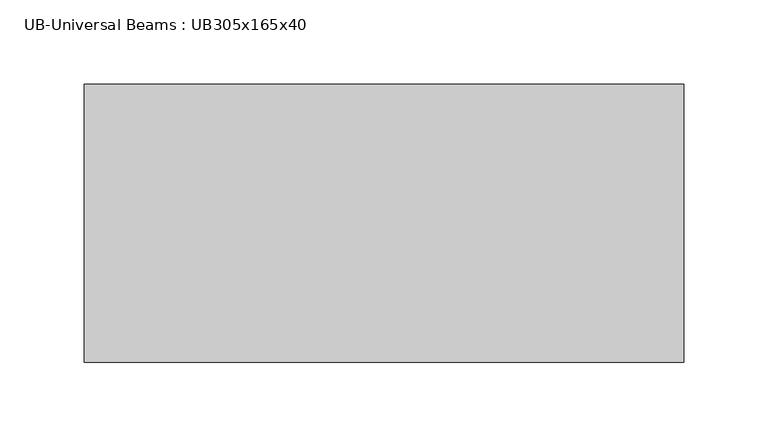
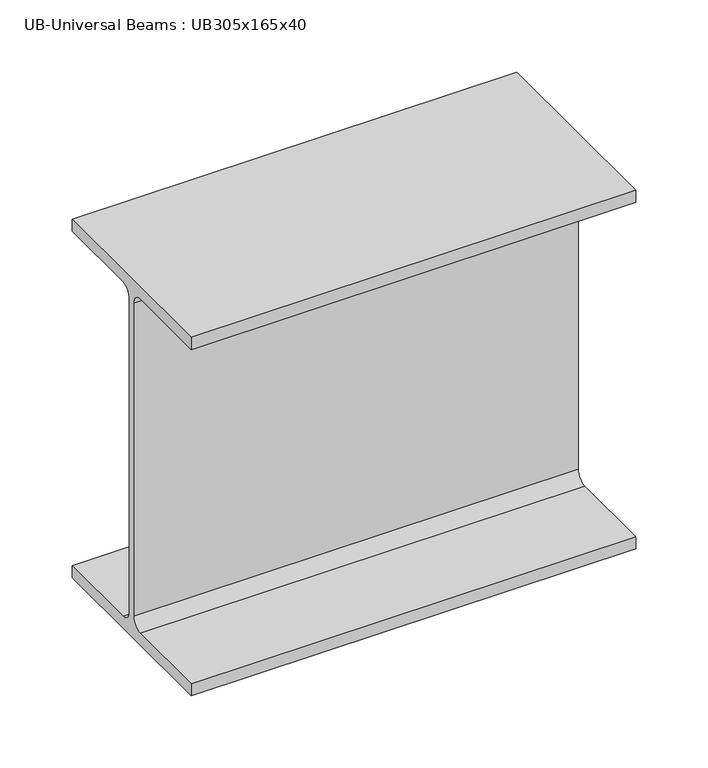
"""IFC4 building model written with IfcOpenShell, lengths in millimetres: beam geometry, UB-Universal Beams : UB305x165x40."""

from ifc_helpers import new_model, si_unit, point, frame, frame_2d, origin, place, context, project, spatial, polyline, circle_curve, trimmed, segment, composite_curve, outline, extrude, source, transform, mapped, element, save


def ub_universal_beams_ub305x165x40_d145b1f7(model_context):
    return source(origin(), model_context, "Body", "SweptSolid", [
        extrude(outline(composite_curve([segment(polyline([(-82.5, -141.5), (-11.9, -141.5)]), True, "CONTINUOUS"), segment(trimmed(circle_curve(frame_2d((-11.9, -132.6)), 8.9), [point((-11.9, -141.5))], [point((-3.0, -132.6))], True, "CARTESIAN"), True, "CONTINUOUS"), segment(polyline([(-3.0, -132.6), (-3.0, 132.6)]), True, "CONTINUOUS"), segment(trimmed(circle_curve(frame_2d((-11.9, 132.6)), 8.9), [point((-3.0, 132.6))], [point((-11.9, 141.5))], True, "CARTESIAN"), True, "CONTINUOUS"), segment(polyline([(-11.9, 141.5), (-82.5, 141.5), (-82.5, 151.7), (82.5, 151.7), (82.5, 141.5), (11.9, 141.5)]), True, "CONTINUOUS"), segment(trimmed(circle_curve(frame_2d((11.9, 132.6)), 8.9), [point((11.9, 141.5))], [point((3.0, 132.6))], True, "CARTESIAN"), True, "CONTINUOUS"), segment(polyline([(3.0, 132.6), (3.0, -132.6)]), True, "CONTINUOUS"), segment(trimmed(circle_curve(frame_2d((11.9, -132.6)), 8.9), [point((3.0, -132.6))], [point((11.9, -141.5))], True, "CARTESIAN"), True, "CONTINUOUS"), segment(polyline([(11.9, -141.5), (82.5, -141.5), (82.5, -151.7), (-82.5, -151.7), (-82.5, -141.5)]), True, "CONTINUOUS")], self_intersect=False)), frame((-665.55, 0.0, 0.0), z_axis=(1.0, 0.0, 0.0), x_axis=(0.0, 1.0, 0.0)), (0.0, 0.0, 1.0), 355.9),
    ])


if __name__ == "__main__":
    model = new_model("IFC4")
    model_context = context("Model", 3, world=origin())
    ifc_project = project(units=[si_unit("LENGTHUNIT", "METRE", prefix="MILLI")], contexts=[model_context])
    site = spatial("IfcSite", under=ifc_project)
    building = spatial("IfcBuilding", under=site)
    placement = place(None, origin())
    ub_universal_beams_ub305x165x40_shape = ub_universal_beams_ub305x165x40_d145b1f7(model_context)
    element("IfcBeam", 1, ObjectType="UB-Universal Beams : UB305x165x40", at=placement, inside=building, context=model_context, shape_type="MappedRepresentation", body=[
        mapped(ub_universal_beams_ub305x165x40_shape, transform((0.0, 0.0, 0.0), x_axis=(1.0, 0.0, 0.0), y_axis=(0.0, 1.0, 0.0), z_axis=(0.0, 0.0, 1.0))),
    ])
    save(model, "model.ifc")

# Revit data of these elements
# Type "UB-Universal Beams : UB305x165x40"
#   Section Name Key = "UB305X165X40"
#   Width = 16.5 cm
#   Web Thickness = 0.6 cm
#   Web Fillet = 0.89 cm
#   Warping Constant = 164000.0 cm⁶
#   Torsional Moment of Inertia = 14.70 cm⁴
#   Section Area = 51.3 cm²
#   Plastic Modulus weak axis = 142.0 cm³
#   Plastic Modulus strong axis = 623.0 cm³
#   Nominal Weight = 40.2999 kgf/m
#   Moment of Inertia weak axis = 764.00 cm⁴
#   Moment of Inertia strong axis = 8503.00 cm⁴
#   Height = 30.34 cm
#   Flange Thickness = 1.02 cm
#   Elastic Modulus weak axis = 92.6 cm³
#   Elastic Modulus strong axis = 560.0 cm³
#   Centroid Vertical = 15.17 cm
#   Centroid Horizontal = 8.25 cm
#   Bolt Spacing = 9.0 cm
#   Length [instance default] = 1500 mm
#   Structural Material [instance default] = Metal - Steel 43-275
#   Type Comments = ""
#   Assembly Code = ""
# Element 1 (IfcBeam, "UB-Universal Beams : UB305x165x40")
#   Materials on its faces: "Metal - Steel 43-275"
# Materials
#   "Metal - Steel 43-275": class "Metal", colour RGB 247 247 247, transparency 0, Cost = 0
